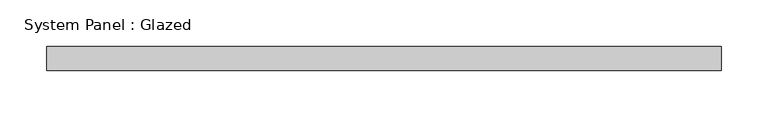
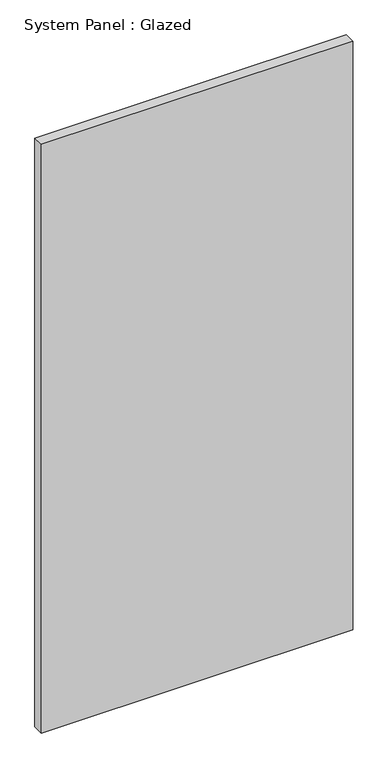
"""IFC4 building model written with IfcOpenShell, lengths in millimetres: plate geometry, System Panel : Glazed."""

from ifc_helpers import new_model, si_unit, origin, origin_with_axes, place, context, project, spatial, polyline, outline, extrude, source, transform, mapped, element, save


def system_panel_glazed_b4a21602(model_context):
    return source(origin(), model_context, "Body", "SweptSolid", [
        extrude(outline(polyline([(358.775, 19.05), (-358.775, 19.05), (-358.775, 44.45), (358.775, 44.45), (358.775, 19.05)])), origin_with_axes(), (0.0, 0.0, 1.0), 1433.9513331),
    ])


if __name__ == "__main__":
    model = new_model("IFC4")
    model_context = context("Model", 3, world=origin())
    ifc_project = project(units=[si_unit("LENGTHUNIT", "METRE", prefix="MILLI")], contexts=[model_context])
    site = spatial("IfcSite", under=ifc_project)
    building = spatial("IfcBuilding", under=site)
    placement = place(None, origin())
    system_panel_glazed_shape = system_panel_glazed_b4a21602(model_context)
    element("IfcPlate", 1, ObjectType="System Panel : Glazed", at=placement, inside=building, context=model_context, shape_type="MappedRepresentation", body=[
        mapped(system_panel_glazed_shape, transform((0.0, 0.0, 0.0), x_axis=(1.0, 0.0, 0.0), y_axis=(0.0, 1.0, 0.0), z_axis=(0.0, 0.0, 1.0))),
    ])
    save(model, "model.ifc")

# Revit data of these elements
# Type "System Panel : Glazed"
#   Construction Type Id = "GSP4R"
#   Analytic Construction = "1/8 in Pilkington single glazing"
#   Visual Light Transmittance = 0.9
#   Solar Heat Gain Coefficient = 0.86
#   Heat Transfer Coefficient (U) = 1.18115 BTU/(h·ft²·°F)
#   Define Thermal Properties by = 1
# Element 1 (IfcPlate, "System Panel : Glazed")
#   Materials on its faces: "Glass"
# Materials
#   "Glass": class "Glass", colour RGB 0 128 192, transparency 0.75, Description = "Soda Lime Glass", Cost = 0
